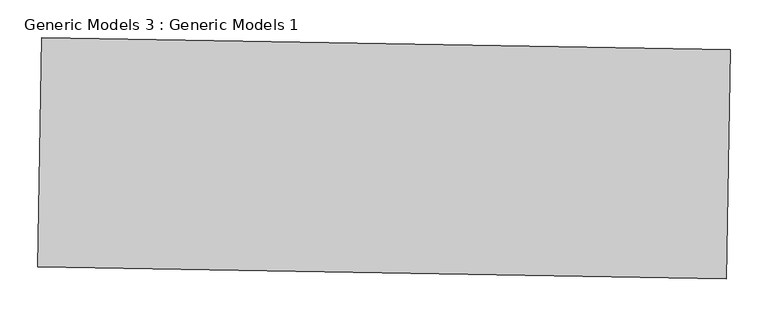
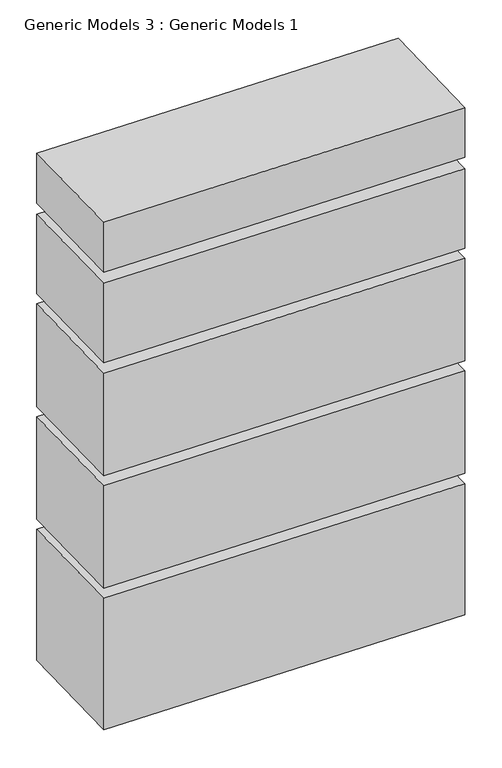
"""IFC4 building model written with IfcOpenShell, lengths in millimetres: proxy geometry, Generic Models 3 : Generic Models 1."""

from ifc_helpers import new_model, si_unit, frame, origin, place, context, project, spatial, polyline, outline, extrude, source, transform, mapped, element, save


def generic_models_3_generic_models_1_5bebd585(model_context):
    return source(origin(), model_context, "Body", "SweptSolid", [
        extrude(outline(polyline([(-1404.2886754, -12512.7515605), (-2318.5494079, -12496.7930801), (-2313.2299144, -12192.0395026), (-1398.969182, -12207.997983), (-1404.2886754, -12512.7515605)])), frame((0.0, 0.0, 1396.5448366), z_axis=(0.0, 0.0, 1.0), x_axis=(1.0, 0.0, 0.0)), (0.0, 0.0, 1.0), 134.9289866),
        extrude(outline(polyline([(-1404.2886754, -12512.7515605), (-2318.5494079, -12496.7930801), (-2313.2299144, -12192.0395026), (-1398.969182, -12207.997983), (-1404.2886754, -12512.7515605)])), frame((0.0, 0.0, 159.8738232), z_axis=(0.0, 0.0, 1.0), x_axis=(1.0, 0.0, 0.0)), (0.0, 0.0, 1.0), 354.4191875),
        extrude(outline(polyline([(-1404.2886754, -12512.7515605), (-2318.5494079, -12496.7930801), (-2313.2299144, -12192.0395026), (-1398.969182, -12207.997983), (-1404.2886754, -12512.7515605)])), frame((0.0, 0.0, 1151.4847196), z_axis=(0.0, 0.0, 1.0), x_axis=(1.0, 0.0, 0.0)), (0.0, 0.0, 1.0), 214.5718039),
        extrude(outline(polyline([(-1404.2886754, -12512.7515605), (-2318.5494079, -12496.7930801), (-2313.2299144, -12192.0395026), (-1398.969182, -12207.997983), (-1404.2886754, -12512.7515605)])), frame((0.0, 0.0, 846.6847196), z_axis=(0.0, 0.0, 1.0), x_axis=(1.0, 0.0, 0.0)), (0.0, 0.0, 1.0), 277.2082911),
        extrude(outline(polyline([(-1404.2886754, -12512.7515605), (-2318.5494079, -12496.7930801), (-2313.2299144, -12192.0395026), (-1398.969182, -12207.997983), (-1404.2886754, -12512.7515605)])), frame((0.0, 0.0, 541.8847196), z_axis=(0.0, 0.0, 1.0), x_axis=(1.0, 0.0, 0.0)), (0.0, 0.0, 1.0), 277.2082911),
    ])


if __name__ == "__main__":
    model = new_model("IFC4")
    model_context = context("Model", 3, world=origin())
    ifc_project = project(units=[si_unit("LENGTHUNIT", "METRE", prefix="MILLI")], contexts=[model_context])
    site = spatial("IfcSite", under=ifc_project)
    building = spatial("IfcBuilding", under=site)
    placement = place(None, origin())
    generic_models_3_generic_models_1_shape = generic_models_3_generic_models_1_5bebd585(model_context)
    element("IfcBuildingElementProxy", 1, Name="Generic Models 3 : Generic Models 1", ObjectType="Generic Models 3 : Generic Models 1", at=placement, inside=building, context=model_context, shape_type="MappedRepresentation", body=[
        mapped(generic_models_3_generic_models_1_shape, transform((0.0, 0.0, 0.0), x_axis=(1.0, 0.0, 0.0), y_axis=(0.0, 1.0, 0.0), z_axis=(0.0, 0.0, 1.0))),
    ])
    save(model, "model.ifc")

# Revit data of these elements
# Element 1 (IfcBuildingElementProxy, "Generic Models 3 : Generic Models 1")
#   Materials on its faces: "Parking Stripe"
# Materials
#   "Parking Stripe": class "Paint", colour RGB 250 250 91, transparency 0, Cost = 0
